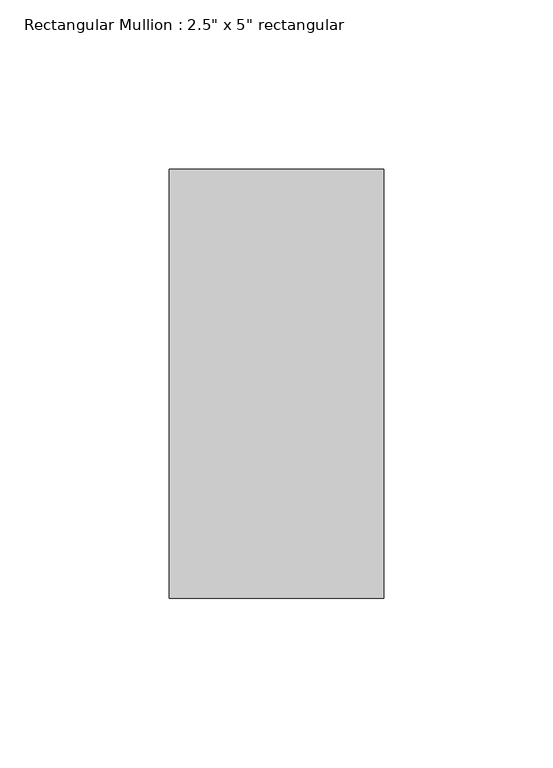
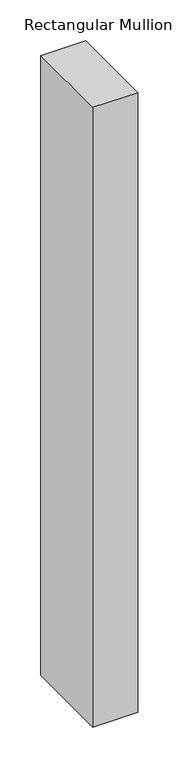
"""IFC4 building model written with IfcOpenShell, lengths in millimetres: member geometry."""

from ifc_helpers import new_model, si_unit, frame, origin, place, context, project, spatial, polyline, outline, extrude, source, transform, mapped, element, save


def member_b689734a(model_context):
    return source(origin(), model_context, "Body", "SweptSolid", [
        extrude(outline(polyline([(31.75, 63.5), (31.75, -63.5), (-31.75, -63.5), (-31.75, 63.5), (31.75, 63.5)])), frame((0.0, 0.0, -924.7594531), z_axis=(0.0, 0.0, 1.0), x_axis=(1.0, 0.0, 0.0)), (0.0, 0.0, 1.0), 924.7594531),
    ])


if __name__ == "__main__":
    model = new_model("IFC4")
    model_context = context("Model", 3, world=origin())
    ifc_project = project(units=[si_unit("LENGTHUNIT", "METRE", prefix="MILLI")], contexts=[model_context])
    site = spatial("IfcSite", under=ifc_project)
    building = spatial("IfcBuilding", under=site)
    placement = place(None, origin())
    member_shape = member_b689734a(model_context)
    element("IfcMember", 1, ObjectType="Rectangular Mullion : 2.5\" x 5\" rectangular", at=placement, inside=building, context=model_context, shape_type="MappedRepresentation", body=[
        mapped(member_shape, transform((0.0, 0.0, 0.0), x_axis=(1.0, 0.0, 0.0), y_axis=(0.0, 1.0, 0.0), z_axis=(0.0, 0.0, 1.0))),
    ])
    save(model, "model.ifc")

# Revit data of these elements
# Type "Rectangular Mullion : 2.5\" x 5\" rectangular"
#   built-in parameter 1007304 = 0.416667 (stored number, unit not read)
#   built-in parameter 1007301 = 0.104167 (stored number, unit not read)
#   built-in parameter 1007300 = 0.104167 (stored number, unit not read)
# Element 1 (IfcMember, "Rectangular Mullion : 2.5\" x 5\" rectangular")
#   Materials on its faces: "Aluminum"
# Materials
#   "Aluminum": class "Metal", colour RGB 247 247 247, transparency 0, Description = "Aluminum 6061", Cost = 0
